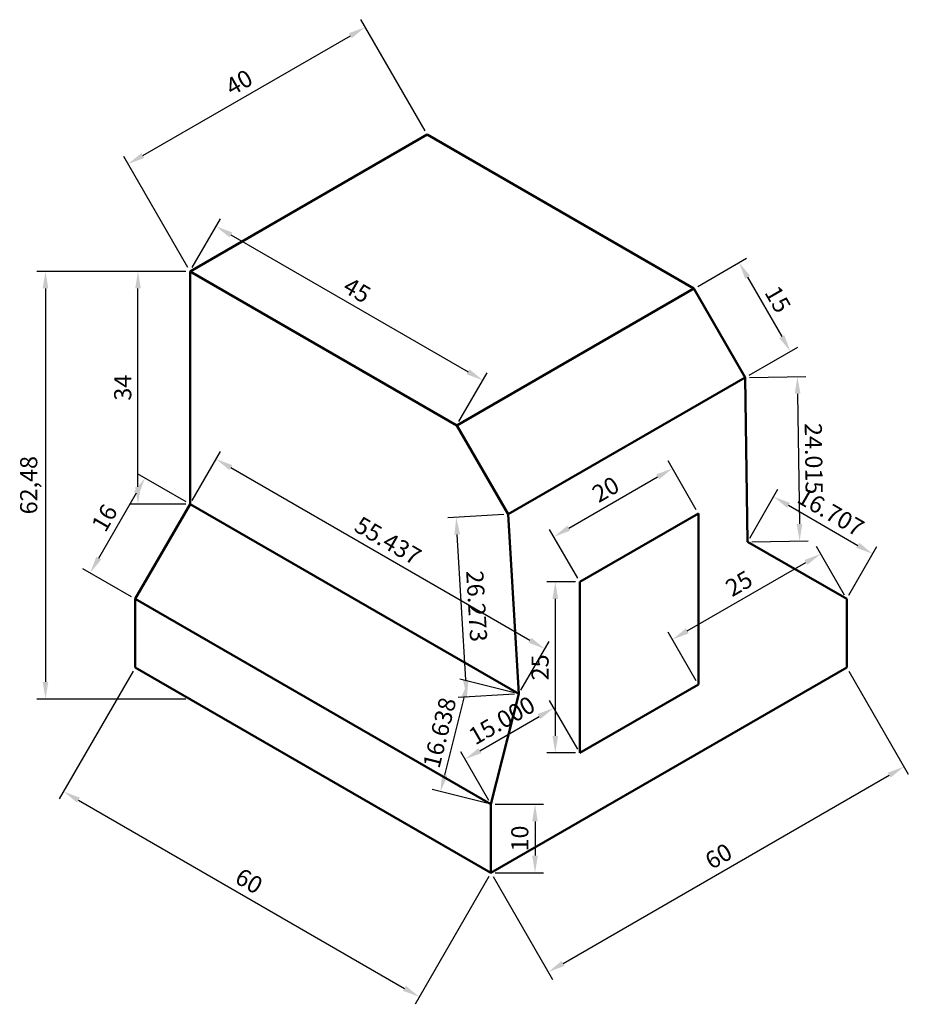
# Model space of a CAD drawing. Units: millimetres. Extents: x 1924 to 2054, y 1132 to 1276.
import ezdxf

# ---------------------------------------------------------------- set-up
doc = ezdxf.new("R2010")
doc.units = ezdxf.units.MM
doc.layers.add('M-DIMS', color=2, linetype='Continuous', lineweight=25)
doc.layers.add('M-OUTL', color=7, linetype='Continuous', lineweight=50)
doc.styles.get("Standard").update_dxf_attribs({"font": 'arial.ttf'})
doc.dimstyles.new('ISO-25', dxfattribs={"dimtxt": 2.5, "dimasz": 2.5, "dimexe": 1.25, "dimexo": 0.625, "dimtad": 1, "dimtxsty": 'Standard', "dimcen": 2.5, "dimadec": 0, "dimazin": 0, "dimtfac": 1, "dimtmove": 0, "dimatfit": 3, "dimfxl": 1, "dimarcsym": 0})

# ---------------------------------------------------------------- blocks, each defined once
blk = doc.blocks.new('*D1')
at = {"layer": 'Defpoints', "color": 0, "transparency": 16777216}
for p in [(2045.27, 1181.15), (2053.64, 1166.65), (1993.31, 1151.15)]:
    blk.add_point(p, dxfattribs=at)
at = {"layer": 'M-DIMS', "color": 0, "lineweight": -2, "transparency": 16777216}
for p, q in [((2045.58, 1180.61), (2054.26, 1165.57)), ((2003.84, 1137.9), (2051.47, 1165.4)), ((1993.62, 1150.61), (2002.3, 1135.57))]:
    blk.add_line(p, q, dxfattribs=at)
at = {"layer": 'M-DIMS', "color": 0, "transparency": 16777216}
for points in [[(2051.27, 1165.76), (2051.68, 1165.04), (2053.64, 1166.65)], [(2003.63, 1138.26), (2004.05, 1137.54), (2001.68, 1136.65)]]:
    blk.add_solid(points, dxfattribs=at)
at = {"layer": 'M-DIMS', "color": 0, "transparency": 16777216, "insert": (2026.71, 1153.29), "char_height": 2.5, "attachment_point": 5, "rotation": 30}
blk.add_mtext('60', dxfattribs=at)
blk = doc.blocks.new('*D2')
at = {"layer": 'Defpoints', "color": 0, "transparency": 16777216}
for p in [(1941.34, 1181.15), (1993.31, 1151.15), (1982.83, 1133.01)]:
    blk.add_point(p, dxfattribs=at)
at = {"layer": 'M-DIMS', "color": 0, "lineweight": -2, "transparency": 16777216}
for p, q in [((1941.03, 1180.61), (1930.25, 1161.93)), ((1933.04, 1161.76), (1980.67, 1134.26)), ((1992.99, 1150.61), (1982.21, 1131.93))]:
    blk.add_line(p, q, dxfattribs=at)
at = {"layer": 'M-DIMS', "color": 0, "transparency": 16777216}
for points in [[(1933.25, 1162.12), (1932.83, 1161.4), (1930.87, 1163.01)], [(1980.88, 1134.62), (1980.46, 1133.9), (1982.83, 1133.01)]]:
    blk.add_solid(points, dxfattribs=at)
at = {"layer": 'M-DIMS', "color": 0, "transparency": 16777216, "insert": (1957.8, 1149.66), "char_height": 2.5, "attachment_point": 5, "rotation": 330}
blk.add_mtext('60', dxfattribs=at)
blk = doc.blocks.new('*D3')
at = {"layer": 'Defpoints', "color": 0, "transparency": 16777216}
for p in [(1949.34, 1239.01), (1928.23, 1176.53), (1949.34, 1176.53)]:
    blk.add_point(p, dxfattribs=at)
at = {"layer": 'M-DIMS', "color": 0, "lineweight": -2, "transparency": 16777216}
for p, q in [((1948.72, 1239.01), (1926.98, 1239.01)), ((1928.23, 1236.51), (1928.23, 1179.03)), ((1948.72, 1176.53), (1926.98, 1176.53))]:
    blk.add_line(p, q, dxfattribs=at)
at = {"layer": 'M-DIMS', "color": 0, "transparency": 16777216}
for points in [[(1927.81, 1236.51), (1928.64, 1236.51), (1928.23, 1239.01)], [(1927.81, 1179.03), (1928.64, 1179.03), (1928.23, 1176.53)]]:
    blk.add_solid(points, dxfattribs=at)
at = {"layer": 'M-DIMS', "color": 0, "transparency": 16777216, "insert": (1926.1, 1207.77), "char_height": 2.5, "attachment_point": 5, "rotation": 90}
blk.add_mtext('62,48', dxfattribs=at)
blk = doc.blocks.new('*D4')
at = {"layer": 'Defpoints', "color": 0, "transparency": 16777216}
for p in [(1974.93, 1274.69), (1983.99, 1259.01), (1949.34, 1239.01)]:
    blk.add_point(p, dxfattribs=at)
at = {"layer": 'M-DIMS', "color": 0, "lineweight": -2, "transparency": 16777216}
for p, q in [((1983.67, 1259.55), (1974.3, 1275.78)), ((1942.45, 1255.94), (1972.76, 1273.44)), ((1949.03, 1239.55), (1939.66, 1255.78))]:
    blk.add_line(p, q, dxfattribs=at)
at = {"layer": 'M-DIMS', "color": 0, "transparency": 16777216}
for points in [[(1972.55, 1273.8), (1972.97, 1273.08), (1974.93, 1274.69)], [(1942.24, 1256.3), (1942.66, 1255.58), (1940.29, 1254.69)]]:
    blk.add_solid(points, dxfattribs=at)
at = {"layer": 'M-DIMS', "color": 0, "transparency": 16777216, "insert": (1956.66, 1266.34), "char_height": 2.5, "attachment_point": 5, "rotation": 30}
blk.add_mtext('40', dxfattribs=at)
blk = doc.blocks.new('*D5')
at = {"layer": 'Defpoints', "color": 0, "transparency": 16777216}
for p in [(2006.3, 1193.65), (2002.7, 1168.65), (2006.3, 1168.65)]:
    blk.add_point(p, dxfattribs=at)
at = {"layer": 'M-DIMS', "color": 0, "lineweight": -2, "transparency": 16777216}
for p, q in [((2005.67, 1193.65), (2001.45, 1193.65)), ((2002.7, 1191.15), (2002.7, 1171.15)), ((2005.67, 1168.65), (2001.45, 1168.65))]:
    blk.add_line(p, q, dxfattribs=at)
at = {"layer": 'M-DIMS', "color": 0, "transparency": 16777216}
for points in [[(2002.28, 1191.15), (2003.11, 1191.15), (2002.7, 1193.65)], [(2002.28, 1171.15), (2003.11, 1171.15), (2002.7, 1168.65)]]:
    blk.add_solid(points, dxfattribs=at)
at = {"layer": 'M-DIMS', "color": 0, "transparency": 16777216, "insert": (2000.8, 1181.15), "char_height": 2.5, "attachment_point": 5, "rotation": 90}
blk.add_mtext('25', dxfattribs=at)
blk = doc.blocks.new('*D6')
at = {"layer": 'Defpoints', "color": 0, "transparency": 16777216}
for p in [(1993.31, 1161.15), (1993.31, 1151.15), (1999.74, 1151.15)]:
    blk.add_point(p, dxfattribs=at)
at = {"layer": 'M-DIMS', "color": 0, "lineweight": -2, "transparency": 16777216}
for p, q in [((1993.93, 1161.15), (2000.99, 1161.15)), ((1999.74, 1158.65), (1999.74, 1153.65)), ((1993.93, 1151.15), (2000.99, 1151.15))]:
    blk.add_line(p, q, dxfattribs=at)
at = {"layer": 'M-DIMS', "color": 0, "transparency": 16777216}
for points in [[(1999.32, 1158.65), (2000.15, 1158.65), (1999.74, 1161.15)], [(1999.32, 1153.65), (2000.15, 1153.65), (1999.74, 1151.15)]]:
    blk.add_solid(points, dxfattribs=at)
at = {"layer": 'M-DIMS', "color": 0, "transparency": 16777216, "insert": (1997.84, 1156.15), "char_height": 2.5, "attachment_point": 5, "rotation": 90}
blk.add_mtext('10', dxfattribs=at)
blk = doc.blocks.new('*D7')
at = {"layer": 'Defpoints', "color": 0, "transparency": 16777216}
for p in [(2019.82, 1210.23), (2023.62, 1203.65), (2006.3, 1193.65)]:
    blk.add_point(p, dxfattribs=at)
at = {"layer": 'M-DIMS', "color": 0, "lineweight": -2, "transparency": 16777216}
for p, q in [((2023.3, 1204.19), (2019.19, 1211.31)), ((2004.66, 1201.48), (2017.65, 1208.98)), ((2005.98, 1194.19), (2001.87, 1201.31))]:
    blk.add_line(p, q, dxfattribs=at)
at = {"layer": 'M-DIMS', "color": 0, "transparency": 16777216}
for points in [[(2017.44, 1209.34), (2017.86, 1208.62), (2019.82, 1210.23)], [(2004.45, 1201.84), (2004.87, 1201.12), (2002.5, 1200.23)]]:
    blk.add_solid(points, dxfattribs=at)
at = {"layer": 'M-DIMS', "color": 0, "transparency": 16777216, "insert": (2010.21, 1206.88), "char_height": 2.5, "attachment_point": 5, "rotation": 30}
blk.add_mtext('20', dxfattribs=at)
blk = doc.blocks.new('*D8')
at = {"layer": 'Defpoints', "color": 0, "transparency": 16777216}
for p in [(2041.47, 1197.73), (2045.27, 1191.15), (2023.62, 1178.65)]:
    blk.add_point(p, dxfattribs=at)
at = {"layer": 'M-DIMS', "color": 0, "lineweight": -2, "transparency": 16777216}
for p, q in [((2044.95, 1191.69), (2040.84, 1198.81)), ((2021.98, 1186.48), (2039.3, 1196.48)), ((2023.3, 1179.19), (2019.19, 1186.31))]:
    blk.add_line(p, q, dxfattribs=at)
at = {"layer": 'M-DIMS', "color": 0, "transparency": 16777216}
for points in [[(2039.09, 1196.84), (2039.51, 1196.12), (2041.47, 1197.73)], [(2021.77, 1186.84), (2022.19, 1186.12), (2019.82, 1185.23)]]:
    blk.add_solid(points, dxfattribs=at)
at = {"layer": 'M-DIMS', "color": 0, "transparency": 16777216, "insert": (2029.69, 1193.13), "char_height": 2.5, "attachment_point": 5, "rotation": 30}
blk.add_mtext('25', dxfattribs=at)
blk = doc.blocks.new('*D9')
at = {"layer": 'Defpoints', "color": 0, "transparency": 16777216}
for p in [(2022.96, 1236.51), (2037.04, 1227.31), (2030.46, 1223.51)]:
    blk.add_point(p, dxfattribs=at)
at = {"layer": 'M-DIMS', "color": 0, "lineweight": -2, "transparency": 16777216}
for p, q in [((2023.5, 1236.82), (2030.62, 1240.93)), ((2030.79, 1238.14), (2035.79, 1229.48)), ((2031, 1223.83), (2038.12, 1227.94))]:
    blk.add_line(p, q, dxfattribs=at)
at = {"layer": 'M-DIMS', "color": 0, "transparency": 16777216}
for points in [[(2031.15, 1238.35), (2030.43, 1237.93), (2029.54, 1240.31)], [(2036.15, 1229.69), (2035.43, 1229.27), (2037.04, 1227.31)]]:
    blk.add_solid(points, dxfattribs=at)
at = {"layer": 'M-DIMS', "color": 0, "transparency": 16777216, "insert": (2034.93, 1234.76), "char_height": 2.5, "attachment_point": 5, "rotation": 300}
blk.add_mtext('15', dxfattribs=at)
blk = doc.blocks.new('*D10')
at = {"layer": 'Defpoints', "color": 0, "transparency": 16777216}
for p in [(1942.76, 1208.81), (1949.34, 1205.01), (1941.34, 1191.15)]:
    blk.add_point(p, dxfattribs=at)
at = {"layer": 'M-DIMS', "color": 0, "lineweight": -2, "transparency": 16777216}
for p, q in [((1948.8, 1205.32), (1941.68, 1209.43)), ((1936.01, 1197.11), (1941.51, 1206.64)), ((1940.8, 1191.46), (1933.68, 1195.57))]:
    blk.add_line(p, q, dxfattribs=at)
at = {"layer": 'M-DIMS', "color": 0, "transparency": 16777216}
for points in [[(1941.15, 1206.85), (1941.87, 1206.43), (1942.76, 1208.81)], [(1935.65, 1197.32), (1936.37, 1196.91), (1934.76, 1194.95)]]:
    blk.add_solid(points, dxfattribs=at)
at = {"layer": 'M-DIMS', "color": 0, "transparency": 16777216, "insert": (1937.12, 1202.83), "char_height": 2.5, "attachment_point": 5, "rotation": 60}
blk.add_mtext('16', dxfattribs=at)
blk = doc.blocks.new('*D11')
at = {"layer": 'Defpoints', "color": 0, "transparency": 16777216}
for p in [(1941.74, 1239.01), (1949.34, 1239.01), (1949.34, 1205.01)]:
    blk.add_point(p, dxfattribs=at)
at = {"layer": 'M-DIMS', "color": 0, "lineweight": -2, "transparency": 16777216}
for p, q in [((1948.72, 1239.01), (1940.49, 1239.01)), ((1941.74, 1207.51), (1941.74, 1236.51)), ((1948.72, 1205.01), (1940.49, 1205.01))]:
    blk.add_line(p, q, dxfattribs=at)
at = {"layer": 'M-DIMS', "color": 0, "transparency": 16777216}
for points in [[(1941.33, 1236.51), (1942.16, 1236.51), (1941.74, 1239.01)], [(1941.33, 1207.51), (1942.16, 1207.51), (1941.74, 1205.01)]]:
    blk.add_solid(points, dxfattribs=at)
at = {"layer": 'M-DIMS', "color": 0, "transparency": 16777216, "insert": (1939.84, 1222.01), "char_height": 2.5, "attachment_point": 5, "rotation": 90}
blk.add_mtext('34', dxfattribs=at)
blk = doc.blocks.new('*D12')
at = {"layer": 'Defpoints', "color": 0, "transparency": 16777216}
for p in [(2030.8, 1199.5), (2049.07, 1197.73), (2045.27, 1191.15)]:
    blk.add_point(p, dxfattribs=at)
at = {"layer": 'M-DIMS', "color": 0, "lineweight": -2, "transparency": 16777216}
for p, q in [((2031.11, 1200.04), (2035.22, 1207.17)), ((2036.76, 1204.83), (2046.9, 1198.98)), ((2045.58, 1191.69), (2049.69, 1198.81))]:
    blk.add_line(p, q, dxfattribs=at)
at = {"layer": 'M-DIMS', "color": 0, "transparency": 16777216}
for points in [[(2036.97, 1205.19), (2036.56, 1204.47), (2034.6, 1206.08)], [(2047.11, 1199.34), (2046.69, 1198.62), (2049.07, 1197.73)]]:
    blk.add_solid(points, dxfattribs=at)
at = {"layer": 'M-DIMS', "color": 0, "transparency": 16777216, "insert": (2042.78, 1203.55), "char_height": 2.5, "attachment_point": 5, "rotation": 330}
blk.add_mtext('16.707', dxfattribs=at)
blk = doc.blocks.new('*D13')
at = {"layer": 'Defpoints', "color": 0, "transparency": 16777216}
for p in [(2030.46, 1223.51), (2030.8, 1199.5), (2038.4, 1199.61)]:
    blk.add_point(p, dxfattribs=at)
at = {"layer": 'M-DIMS', "color": 0, "lineweight": -2, "transparency": 16777216}
for p, q in [((2031.08, 1223.52), (2039.31, 1223.64)), ((2038.09, 1221.12), (2038.36, 1202.11)), ((2031.42, 1199.51), (2039.65, 1199.63))]:
    blk.add_line(p, q, dxfattribs=at)
at = {"layer": 'M-DIMS', "color": 0, "transparency": 16777216}
for points in [[(2038.51, 1221.13), (2037.67, 1221.12), (2038.06, 1223.62)], [(2038.78, 1202.12), (2037.95, 1202.1), (2038.4, 1199.61)]]:
    blk.add_solid(points, dxfattribs=at)
at = {"layer": 'M-DIMS', "color": 0, "transparency": 16777216, "insert": (2040.13, 1211.64), "char_height": 2.5, "attachment_point": 5, "rotation": 270.8175}
blk.add_mtext('24.015', dxfattribs=at)
blk = doc.blocks.new('*D14')
at = {"layer": 'Defpoints', "color": 0, "transparency": 16777216}
for p in [(1949.34, 1239.01), (1992.12, 1223.09), (1988.32, 1216.51)]:
    blk.add_point(p, dxfattribs=at)
at = {"layer": 'M-DIMS', "color": 0, "lineweight": -2, "transparency": 16777216}
for p, q in [((1949.66, 1239.55), (1953.77, 1246.67)), ((1955.31, 1244.34), (1989.95, 1224.34)), ((1988.63, 1217.05), (1992.74, 1224.17))]:
    blk.add_line(p, q, dxfattribs=at)
at = {"layer": 'M-DIMS', "color": 0, "transparency": 16777216}
for points in [[(1955.52, 1244.7), (1955.1, 1243.98), (1953.14, 1245.59)], [(1990.16, 1224.7), (1989.74, 1223.98), (1992.12, 1223.09)]]:
    blk.add_solid(points, dxfattribs=at)
at = {"layer": 'M-DIMS', "color": 0, "transparency": 16777216, "insert": (1973.58, 1235.98), "char_height": 2.5, "attachment_point": 5, "rotation": 330}
blk.add_mtext('45', dxfattribs=at)
blk = doc.blocks.new('*D15')
at = {"layer": 'Defpoints', "color": 0, "transparency": 16777216}
for p in [(1988.23, 1203.07), (1995.82, 1203.51), (1997.35, 1177.29)]:
    blk.add_point(p, dxfattribs=at)
at = {"layer": 'M-DIMS', "color": 0, "lineweight": -2, "transparency": 16777216}
for p, q in [((1995.19, 1203.48), (1986.98, 1203)), ((1989.62, 1179.34), (1988.37, 1200.57)), ((1996.73, 1177.25), (1988.52, 1176.77))]:
    blk.add_line(p, q, dxfattribs=at)
at = {"layer": 'M-DIMS', "color": 0, "transparency": 16777216}
for points in [[(1988.79, 1200.6), (1987.96, 1200.55), (1988.23, 1203.07)], [(1990.04, 1179.36), (1989.21, 1179.31), (1989.77, 1176.84)]]:
    blk.add_solid(points, dxfattribs=at)
at = {"layer": 'M-DIMS', "color": 0, "transparency": 16777216, "insert": (1990.9, 1190.07), "char_height": 2.5, "attachment_point": 5, "rotation": 273.3584}
blk.add_mtext('26.273', dxfattribs=at)
blk = doc.blocks.new('*D16')
at = {"layer": 'Defpoints', "color": 0, "transparency": 16777216}
for p in [(1989.98, 1179.14), (1997.35, 1177.29), (1993.31, 1161.15)]:
    blk.add_point(p, dxfattribs=at)
at = {"layer": 'M-DIMS', "color": 0, "lineweight": -2, "transparency": 16777216}
for p, q in [((1996.75, 1177.44), (1988.77, 1179.44)), ((1986.54, 1165.42), (1989.37, 1176.71)), ((1992.7, 1161.3), (1984.72, 1163.3))]:
    blk.add_line(p, q, dxfattribs=at)
at = {"layer": 'M-DIMS', "color": 0, "transparency": 16777216}
for points in [[(1988.97, 1176.81), (1989.78, 1176.61), (1989.98, 1179.14)], [(1986.14, 1165.52), (1986.95, 1165.32), (1985.93, 1163)]]:
    blk.add_solid(points, dxfattribs=at)
at = {"layer": 'M-DIMS', "color": 0, "transparency": 16777216, "insert": (1986.11, 1171.53), "char_height": 2.5, "attachment_point": 5, "rotation": 75.9159}
blk.add_mtext('16.638', dxfattribs=at)
blk = doc.blocks.new('*D17')
at = {"layer": 'Defpoints', "color": 0, "transparency": 16777216}
for p in [(2002.5, 1175.23), (2006.3, 1168.65), (1993.31, 1161.15)]:
    blk.add_point(p, dxfattribs=at)
at = {"layer": 'M-DIMS', "color": 0, "lineweight": -2, "transparency": 16777216}
for p, q in [((2005.98, 1169.19), (2001.87, 1176.31)), ((1991.67, 1168.98), (2000.33, 1173.98)), ((1992.99, 1161.69), (1988.88, 1168.81))]:
    blk.add_line(p, q, dxfattribs=at)
at = {"layer": 'M-DIMS', "color": 0, "transparency": 16777216}
for points in [[(2000.12, 1174.34), (2000.54, 1173.62), (2002.5, 1175.23)], [(1991.46, 1169.34), (1991.88, 1168.62), (1989.51, 1167.73)]]:
    blk.add_solid(points, dxfattribs=at)
at = {"layer": 'M-DIMS', "color": 0, "transparency": 16777216, "insert": (1995.05, 1173.13), "char_height": 2.5, "attachment_point": 5, "rotation": 30}
blk.add_mtext('15.000', dxfattribs=at)
blk = doc.blocks.new('*D18')
at = {"layer": 'Defpoints', "color": 0, "transparency": 16777216}
for p in [(1949.34, 1205.01), (2001.15, 1183.87), (1997.35, 1177.29)]:
    blk.add_point(p, dxfattribs=at)
at = {"layer": 'M-DIMS', "color": 0, "lineweight": -2, "transparency": 16777216}
for p, q in [((1949.66, 1205.55), (1953.77, 1212.67)), ((1955.31, 1210.34), (1998.99, 1185.12)), ((1997.67, 1177.83), (2001.78, 1184.95))]:
    blk.add_line(p, q, dxfattribs=at)
at = {"layer": 'M-DIMS', "color": 0, "transparency": 16777216}
for points in [[(1955.52, 1210.7), (1955.1, 1209.98), (1953.14, 1211.59)], [(1999.2, 1185.48), (1998.78, 1184.76), (2001.15, 1183.87)]]:
    blk.add_solid(points, dxfattribs=at)
at = {"layer": 'M-DIMS', "color": 0, "transparency": 16777216, "insert": (1978.1, 1199.38), "char_height": 2.5, "attachment_point": 5, "rotation": 330}
blk.add_mtext('55.437', dxfattribs=at)

msp = doc.modelspace()

# ---------------------------------------------------------------- linework, layer by layer
at = {"layer": 'M-OUTL'}
for p, q in [((1949.3441, 1239.0052), (1983.9851, 1259.0052)), ((1983.9851, 1259.0052), (2022.9563, 1236.5052)), ((1949.3441, 1205.0052), (1949.3441, 1239.0052)), ((1988.3153, 1216.5052), (1949.3441, 1239.0052)), ((2022.9563, 1236.5052), (1988.3153, 1216.5052)), ((2022.9563, 1236.5052), (2030.4563, 1223.5148)), ((1995.8153, 1203.5148), (2030.4563, 1223.5148)), ((2030.4563, 1223.5148), (2030.7989, 1199.502)), ((1988.3153, 1216.5052), (1995.8153, 1203.5148)), ((1941.3441, 1191.1488), (1949.3441, 1205.0052)), ((1949.3441, 1205.0052), (1997.3544, 1177.2865)), ((1995.8153, 1203.5148), (1997.3544, 1177.2865)), ((2006.296, 1193.6488), (2023.6165, 1203.6488)), ((2023.6165, 1203.6488), (2023.6165, 1178.6488)), ((2045.2672, 1191.1488), (2030.7989, 1199.502)), ((2006.296, 1168.6488), (2006.296, 1193.6488)), ((1941.3441, 1181.1488), (1941.3441, 1191.1488)), ((1941.3441, 1191.1488), (1993.3057, 1161.1488)), ((2045.2672, 1181.1488), (2045.2672, 1191.1488)), ((1993.3057, 1151.1488), (1941.3441, 1181.1488)), ((1993.3057, 1151.1488), (2045.2672, 1181.1488)), ((2023.6165, 1178.6488), (2006.296, 1168.6488)), ((1993.3057, 1161.1488), (1997.3544, 1177.2865)), ((1993.3057, 1161.1488), (1993.3057, 1151.1488))]:
    msp.add_line(p, q, dxfattribs=at)

# ---------------------------------------------------------------- dimensions: what is measured, and where the dimension line sits
at = {"layer": 'M-DIMS'}
for p1, p2, distance, picture, middle in [((1949.3441, 1239.0052), (1983.9851, 1259.0052), 18.1155, '*D4', (1956.6562, 1266.3404)), ((1949.3441, 1239.0052), (1949.3441, 1176.53), -21.1159, '*D3', (1926.1009, 1207.7676)), ((2006.296, 1193.6488), (2006.296, 1168.6488), -3.5989, '*D5', (2000.7957, 1181.1488)), ((1941.3441, 1181.1488), (1993.3057, 1151.1488), -20.9443, '*D2', (1957.8035, 1149.6572)), ((1993.3057, 1151.1488), (2045.2672, 1181.1488), -16.7446, '*D1', (2026.708, 1153.2942)), ((1993.3057, 1161.1488), (1993.3057, 1151.1488), 6.4314, '*D6', (1997.8356, 1156.1488))]:
    dim = msp.add_aligned_dim(p1=p1, p2=p2, distance=distance, dimstyle='ISO-25', override={"dimclrd": 0, "dimclre": 0, "dimclrt": 0}, dxfattribs=at)
    dim.commit()
    dim.dimension.update_dxf_attribs({"geometry": picture, "text_midpoint": middle})
for base, p1, p2, angle, override, picture, middle in [((1992.1153, 1223.087), (1949.3441, 1239.0052), (1988.3153, 1216.5052), 330, {"dimdec": 0, "dimlfac": 1, "dimrnd": 0, "dimzin": 0, "dimdsep": 46, "dimlunit": 2}, '*D14', (1973.5779, 1235.9792)), ((2037.0381, 1227.3148), (2022.9563, 1236.5052), (2030.4563, 1223.5148), 300, {"dimdec": 0, "dimlfac": 1, "dimrnd": 0, "dimzin": 0, "dimdsep": 46, "dimlunit": 2}, '*D9', (2034.9348, 1234.7607)), ((1941.7441, 1239.0052), (1949.3441, 1205.0052), (1949.3441, 1239.0052), 90, {"dimdec": 0, "dimlfac": 1, "dimrnd": 0, "dimzin": 0, "dimdsep": 46, "dimlunit": 2}, '*D11', (1939.8418, 1222.0052)), ((2038.3981, 1199.6105), (2030.4563, 1223.5148), (2030.7989, 1199.502), 270.817479, {"dimdec": 3, "dimlfac": 1, "dimrnd": 0, "dimzin": 0, "dimdsep": 46, "dimlunit": 2}, '*D13', (2040.1281, 1211.644)), ((2001.1544, 1183.8682), (1949.3441, 1205.0052), (1997.3544, 1177.2865), 330, {"dimdec": 3, "dimlfac": 1, "dimrnd": 0, "dimzin": 0, "dimdsep": 46, "dimlunit": 2}, '*D18', (1978.1004, 1199.375)), ((2019.8165, 1210.2306), (2006.296, 1193.6488), (2023.6165, 1203.6488), 30, {"dimdec": 0, "dimlfac": 1, "dimrnd": 0, "dimzin": 0, "dimdsep": 46, "dimlunit": 2}, '*D7', (2010.2056, 1206.8773)), ((1942.7623, 1208.8052), (1941.3441, 1191.1488), (1949.3441, 1205.0052), 60, {"dimdec": 0, "dimlfac": 1, "dimrnd": 0, "dimzin": 0, "dimdsep": 46, "dimlunit": 2}, '*D10', (1937.1156, 1202.8277)), ((2049.0672, 1197.7306), (2030.7989, 1199.502), (2045.2672, 1191.1488), 330, {"dimdec": 3, "dimlfac": 1, "dimrnd": 0, "dimzin": 0, "dimdsep": 46, "dimlunit": 2}, '*D12', (2042.7838, 1203.5539)), ((1988.2283, 1203.0696), (1997.3544, 1177.2865), (1995.8153, 1203.5148), 93.358371, {"dimdec": 3, "dimlfac": 1, "dimrnd": 0, "dimzin": 0, "dimdsep": 46, "dimlunit": 2}, '*D15', (1990.8969, 1190.0669)), ((2041.4672, 1197.7306), (2023.6165, 1178.6488), (2045.2672, 1191.1488), 30, {"dimdec": 0, "dimlfac": 1, "dimrnd": 0, "dimzin": 0, "dimdsep": 46, "dimlunit": 2}, '*D8', (2029.6911, 1193.1273)), ((1989.9829, 1179.1359), (1993.3057, 1161.1488), (1997.3544, 1177.2865), 75.915875, {"dimdec": 3, "dimlfac": 1, "dimrnd": 0, "dimzin": 0, "dimdsep": 46, "dimlunit": 2}, '*D16', (1986.1134, 1171.53)), ((2002.496, 1175.2306), (1993.3057, 1161.1488), (2006.296, 1168.6488), 30, {"dimdec": 3, "dimlfac": 1, "dimrnd": 0, "dimzin": 0, "dimdsep": 46, "dimlunit": 2}, '*D17', (1995.0501, 1173.1273))]:
    dim = msp.add_linear_dim(base=base, p1=p1, p2=p2, angle=angle, dimstyle='ISO-25', override=override, dxfattribs=at)
    dim.commit()
    dim.dimension.update_dxf_attribs({"geometry": picture, "text_midpoint": middle})

doc.saveas('drawing.dxf')
